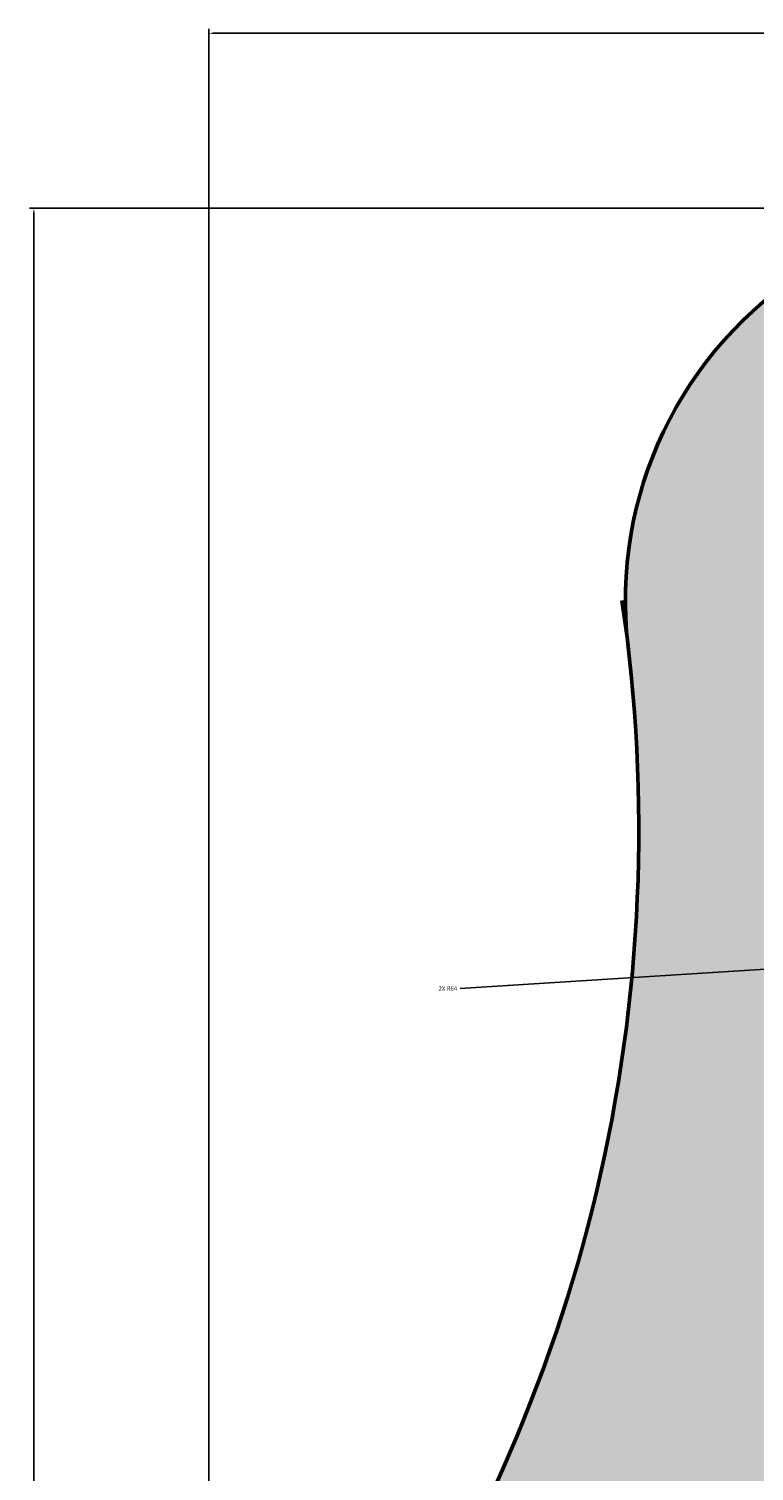
# Model space of a CAD drawing. Units: inches. Extents: x -13 to 107, y -48 to 102.
# Tile 10 of 13: x -13 to 17, y 43 to 102. Entities that reach past the tile are written whole.
import ezdxf

# ---------------------------------------------------------------- set-up
doc = ezdxf.new("R2010")
doc.units = ezdxf.units.IN
doc.header["$MEASUREMENT"] = 0
for name, color, linetype, lineweight in [('M-DIMS', 2, 'Continuous', 18), ('M-HATC', 8, 'Continuous', 18), ('M-OUTL', 7, 'Continuous', 50)]:
    doc.layers.add(name, color=color, linetype=linetype, lineweight=lineweight)
doc.styles.get("Standard").update_dxf_attribs({"font": 'arial.ttf'})
doc.dimstyles.get("Standard").update_dxf_attribs({"dimtxt": 0.18, "dimasz": 0.18, "dimexe": 0.18, "dimexo": 0.0625, "dimgap": 0.09, "dimtad": 0, "dimtih": 1, "dimtoh": 1, "dimdec": 4, "dimzin": 0, "dimdsep": 46, "dimtxsty": 'Standard', "dimcen": 0.09, "dimadec": 0, "dimazin": 0, "dimtfac": 1, "dimtdec": 4, "dimtofl": 0, "dimtmove": 0, "dimatfit": 3, "dimfxl": 1, "dimtolj": 1, "dimtzin": 0, "dimarcsym": 0})

# ---------------------------------------------------------------- blocks, each defined once
blk = doc.blocks.new('*D1')
at = {"layer": 'Defpoints', "color": 0, "transparency": 16777216}
for p in [(60.544, 101.543), (-5.45, 13.883), (60.544, 13.883)]:
    blk.add_point(p, dxfattribs=at)
at = {"layer": 'M-DIMS', "color": 0, "lineweight": -2, "transparency": 16777216}
for p, q in [((-5.45, 13.945), (-5.45, 101.723)), ((-5.27, 101.543), (27.328, 101.543)), ((60.364, 101.543), (27.766, 101.543)), ((60.544, 13.945), (60.544, 101.723))]:
    blk.add_line(p, q, dxfattribs=at)
at = {"layer": 'M-DIMS', "color": 0, "transparency": 16777216}
for points in [[(-5.27, 101.573), (-5.27, 101.513), (-5.45, 101.543)], [(60.364, 101.573), (60.364, 101.513), (60.544, 101.543)]]:
    blk.add_solid(points, dxfattribs=at)
at = {"layer": 'M-DIMS', "color": 0, "transparency": 16777216, "insert": (27.547, 101.543), "char_height": 0.18, "attachment_point": 5}
blk.add_mtext('\\A1;66', dxfattribs=at)
blk = doc.blocks.new('*D2')
at = {"layer": 'Defpoints', "color": 0, "transparency": 16777216}
for p in [(-12.585, 94.408), (27.547, 94.408), (27.547, -46.592)]:
    blk.add_point(p, dxfattribs=at)
at = {"layer": 'M-DIMS', "color": 0, "lineweight": -2, "transparency": 16777216}
for p, q in [((27.484, 94.408), (-12.765, 94.408)), ((-12.585, 94.228), (-12.585, 24.088)), ((-12.585, -46.412), (-12.585, 23.727)), ((27.484, -46.592), (-12.765, -46.592))]:
    blk.add_line(p, q, dxfattribs=at)
at = {"layer": 'M-DIMS', "color": 0, "transparency": 16777216}
for points in [[(-12.615, 94.228), (-12.555, 94.228), (-12.585, 94.408)], [(-12.615, -46.412), (-12.555, -46.412), (-12.585, -46.592)]]:
    blk.add_solid(points, dxfattribs=at)
at = {"layer": 'M-DIMS', "color": 0, "transparency": 16777216, "insert": (-12.585, 23.908), "char_height": 0.18, "attachment_point": 5}
blk.add_mtext('\\A1;141', dxfattribs=at)
blk = doc.blocks.new('*D14')
at = {"layer": 'Defpoints', "color": 0, "transparency": 16777216}
for p in [(106.998, 69.054), (43.126, 65.005)]:
    blk.add_point(p, dxfattribs=at)
at = {"layer": 'M-DIMS', "color": 0, "lineweight": -2, "transparency": 16777216}
for p, q in [((106.908, 69.054), (107.088, 69.054)), ((106.998, 68.964), (106.998, 69.144)), ((4.803, 62.576), (42.947, 64.994))]:
    blk.add_line(p, q, dxfattribs=at)
at = {"layer": 'M-DIMS', "color": 0, "transparency": 16777216}
blk.add_solid([(42.945, 65.024), (42.949, 64.964), (43.126, 65.005)], dxfattribs=at)
at = {"layer": 'M-DIMS', "color": 0, "transparency": 16777216, "insert": (4.304, 62.576), "char_height": 0.18, "attachment_point": 5}
blk.add_mtext('\\A1;2X R64', dxfattribs=at)

msp = doc.modelspace()

# ---------------------------------------------------------------- hatches: boundary and pattern name
at = {"layer": 'M-HATC'}
h = msp.add_hatch(color=256, dxfattribs=at)
h.set_gradient(color1=(88, 186, 72), color2=(241, 235, 31), tint=1)
h.paths.add_polyline_path([(45.86, -14.044, 0.420873), (54.577, 32.339, -0.184081), (43.437, 76.537, 1.124637), (11.657, 76.537, -0.184081), (0.517, 32.339, 0.420873), (9.234, -14.044, -0.304084), (17.743, -34.622, 1.220926), (37.351, -34.622, -0.304084)])
h.paths.add_polyline_path([(33.479, -5.692, 0.859727), (21.615, -5.692, -0.111692), (13.972, -1.28, 0.859727), (8.04, 8.995, -0.111692), (8.04, 17.82, 0.859727), (13.972, 28.095, -0.111692), (21.615, 32.508, 0.859727), (33.479, 32.508, -0.111692), (41.122, 28.095, 0.859727), (47.054, 17.82, -0.111692), (47.054, 8.995, 0.859727), (41.122, -1.28, -0.111692)], flags=16)
h.paths.add_polyline_path([(32.547, -36.592, -1), (22.547, -36.592, -1)], flags=16)
h.paths.add_polyline_path([(17.547, 78.408, -1), (37.547, 78.408, -1)], flags=16)

# ---------------------------------------------------------------- linework, layer by layer
at = {"layer": 'M-OUTL'}
for centre, radius, start, end in [((27.547, 78.408), 16, 353.28544, 186.71456), ((-51.904, 69.054), 64, 324.99334, 8.4041)]:
    msp.add_arc(centre, radius, start, end, dxfattribs=at)

# ---------------------------------------------------------------- dimensions: what is measured, and where the dimension line sits
at = {"layer": 'M-DIMS'}
dim = msp.add_linear_dim(base=(60.544, 101.543), p1=(-5.45, 13.883), p2=(60.544, 13.883), dimstyle='Standard', override={"dimdec": 0, "dimlfac": 1, "dimrnd": 0, "dimzin": 0, "dimdsep": 46, "dimlunit": 2}, dxfattribs=at)
dim.commit()
dim.dimension.update_dxf_attribs({"geometry": '*D1', "text_midpoint": (27.547, 101.543)})
dim = msp.add_linear_dim(base=(-12.585, 94.408), p1=(27.547, -46.592), p2=(27.547, 94.408), angle=90, dimstyle='Standard', override={"dimdec": 0, "dimlfac": 1, "dimrnd": 0, "dimzin": 0, "dimdsep": 46, "dimlunit": 2}, dxfattribs=at)
dim.commit()
dim.dimension.update_dxf_attribs({"geometry": '*D2', "text_midpoint": (-12.585, 23.908)})
dim = msp.add_radius_dim(center=(106.998, 69.054), mpoint=(43.126, 65.005), text='2X <>', dimstyle='Standard', override={"dimdec": 0, "dimlfac": 1, "dimrnd": 0, "dimzin": 0, "dimdsep": 46, "dimlunit": 2}, dxfattribs=at)
dim.commit()
dim.dimension.update_dxf_attribs({"geometry": '*D14', "text_midpoint": (4.803, 62.576), "dimtype": 164})

doc.saveas('drawing.dxf')
